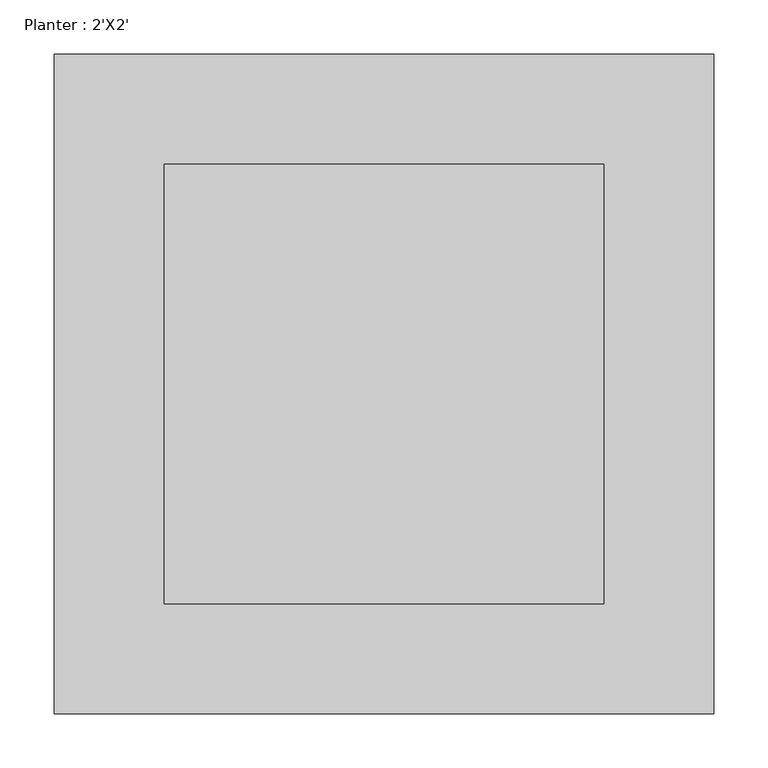
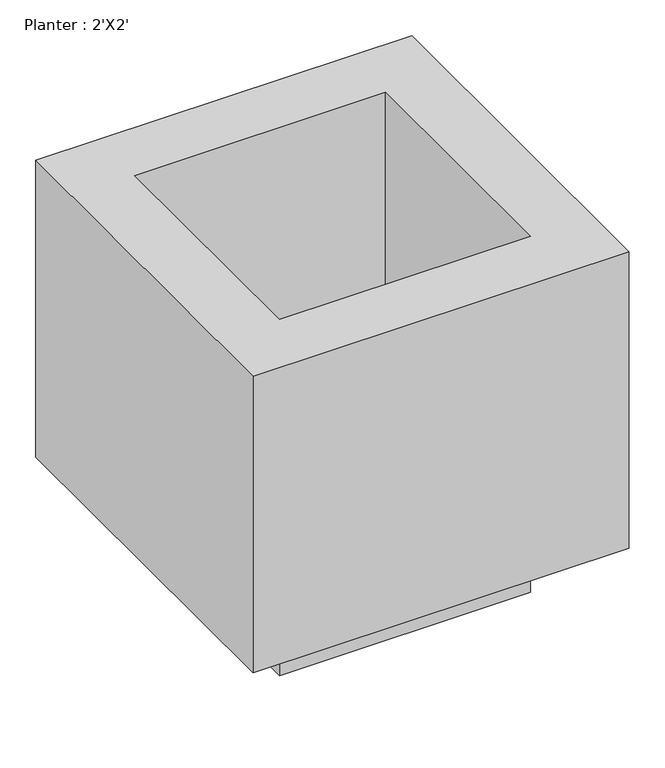
"""IFC4 building model written with IfcOpenShell, lengths in millimetres: geographic element geometry, Planter : 2'X2'."""

from ifc_helpers import new_model, si_unit, origin, origin_with_axes, place, context, project, spatial, polyline, outline, extrude, faceted_brep, source, transform, mapped, element, save


def planter_2_x2_da431093(model_context):
    return source(origin(), model_context, "Body", "SolidModel", [
        faceted_brep([(304.8, 304.8, 609.6), (-304.8, 304.8, 609.6), (-304.8, -304.8, 609.6), (304.8, -304.8, 609.6), (-203.2, 203.2, 609.6), (203.2, 203.2, 609.6), (203.2, -203.2, 609.6), (-203.2, -203.2, 609.6), (304.8, 304.8, 101.6), (304.8, -304.8, 101.6), (-304.8, -304.8, 101.6), (-304.8, 304.8, 101.6), (203.2, 203.2, 203.2), (-203.2, 203.2, 203.2), (-203.2, -203.2, 203.2), (203.2, -203.2, 203.2)], [[[0, 1, 2, 3], [4, 5, 6, 7]], [[8, 9, 10, 11]], [[1, 0, 8, 11]], [[2, 1, 11, 10]], [[3, 2, 10, 9]], [[0, 3, 9, 8]], [[12, 13, 14, 15]], [[13, 12, 5, 4]], [[14, 13, 4, 7]], [[15, 14, 7, 6]], [[12, 15, 6, 5]]]),
        extrude(outline(polyline([(203.2, 203.2), (203.2, -203.2), (-203.2, -203.2), (-203.2, 203.2), (203.2, 203.2)])), origin_with_axes(), (0.0, 0.0, 1.0), 101.6),
    ])


if __name__ == "__main__":
    model = new_model("IFC4")
    model_context = context("Model", 3, world=origin())
    ifc_project = project(units=[si_unit("LENGTHUNIT", "METRE", prefix="MILLI")], contexts=[model_context])
    site = spatial("IfcSite", under=ifc_project)
    building = spatial("IfcBuilding", under=site)
    placement = place(None, origin())
    planter_2_x2_shape = planter_2_x2_da431093(model_context)
    element("IfcGeographicElement", 1, ObjectType="Planter : 2'X2'", at=placement, inside=building, context=model_context, shape_type="MappedRepresentation", body=[
        mapped(planter_2_x2_shape, transform((0.0, 0.0, 0.0), x_axis=(1.0, 0.0, 0.0), y_axis=(0.0, 1.0, 0.0), z_axis=(0.0, 0.0, 1.0))),
    ])
    save(model, "model.ifc")

# Revit data of these elements
# Type "Planter : 2'X2'"
#   Depth = 2' - 0"
#   Height = 2' - 0"
#   Width = 2' - 0"
#   Material = Concrete, Precast
# Element 1 (IfcGeographicElement, "Planter : 2'X2'")
#   Materials on its faces: "Concrete, Precast"
# Materials
#   "Concrete, Precast": class "Concrete", colour RGB 198 187 187, transparency 0, Description = "Precast concrete", Cost = 0
